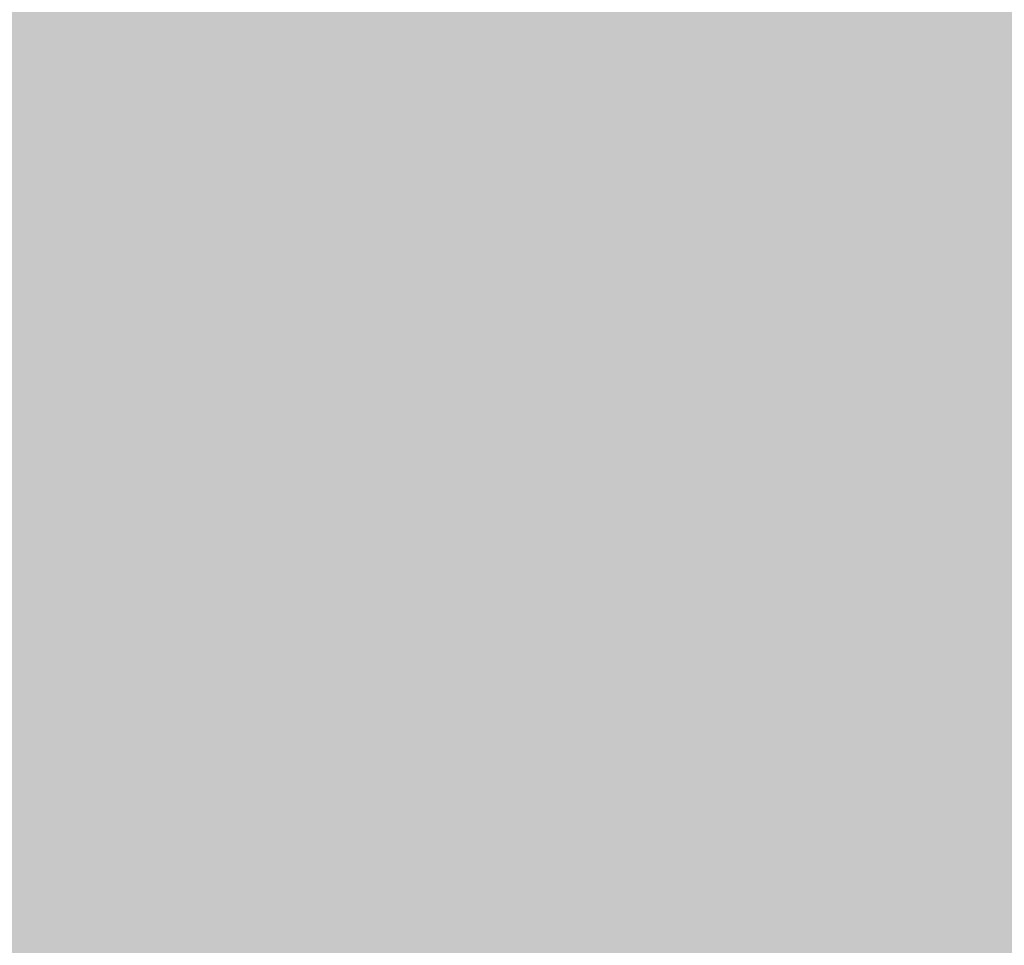
# Model space of a CAD drawing. Units: millimetres. Extents: x -22994 to 29398, y -19990 to 20176.
# Tile 86 of 135: x 227.437 to 229.428, y 85.199 to 87.071. Entities that reach past the tile are written whole.
import ezdxf
from ezdxf import colors
from ezdxf.entities.mleader import LeaderData, LeaderLine
from ezdxf.math import Vec2, Vec3

# ---------------------------------------------------------------- set-up
doc = ezdxf.new("R2010")
doc.units = ezdxf.units.MM
doc.header["$MEASUREMENT"] = 0
doc.layers.add('M-ANNO-TEXT', color=7, linetype='Continuous', lineweight=25)
doc.layers.add('M-DIMS', color=2, linetype='Continuous', lineweight=18)
doc.styles.get("Standard").update_dxf_attribs({"font": 'arial.ttf'})
doc.dimstyles.get("Standard").update_dxf_attribs({"dimtxt": 0.18, "dimasz": 10000, "dimexe": 0.18, "dimexo": 0.0625, "dimgap": 0.09, "dimtad": 0, "dimtih": 1, "dimtoh": 1, "dimdec": 0, "dimzin": 0, "dimdsep": 46, "dimtxsty": 'Standard', "dimcen": 0.09, "dimadec": 0, "dimazin": 0, "dimtfac": 1, "dimtdec": 0, "dimtofl": 0, "dimtmove": 0, "dimatfit": 3, "dimfxl": 1, "dimtolj": 1, "dimtzin": 0, "dimlwd": 30, "dimarcsym": 0})

# ---------------------------------------------------------------- blocks, each defined once
blk = doc.blocks.new('*D2')
at = {"layer": 'Defpoints', "color": 0, "transparency": 16777216}
for p in [(6.6773, 10.2713), (290.852, 10.2713), (290.852, -5.0787)]:
    blk.add_point(p, dxfattribs=at)
at = {"layer": 'M-DIMS', "color": 0, "lineweight": -2, "transparency": 16777216}
for p, q in [((6.6773, 10.2088), (6.6773, -5.2587)), ((290.852, 10.2088), (290.852, -5.2587))]:
    blk.add_line(p, q, dxfattribs=at)
at = {"layer": 'M-DIMS', "color": 0, "lineweight": 30, "transparency": 16777216}
for p, q in [((-9993.3227, -5.0787), (-19993.3227, -5.0787)), ((10290.852, -5.0787), (20290.852, -5.0787))]:
    blk.add_line(p, q, dxfattribs=at)
at = {"layer": 'M-DIMS', "color": 0, "transparency": 16777216}
for points in [[(-9993.3227, 1661.5879), (-9993.3227, -1671.7454), (6.6773, -5.0787)], [(10290.852, 1661.5879), (10290.852, -1671.7454), (290.852, -5.0787)]]:
    blk.add_solid(points, dxfattribs=at)
at = {"layer": 'M-DIMS', "color": 0, "transparency": 16777216, "insert": (148.7647, -5.0787), "char_height": 0.18, "attachment_point": 5}
blk.add_mtext('\\A1;284.2', dxfattribs=at)
blk = doc.blocks.new('*D3')
at = {"layer": 'Defpoints', "color": 0, "transparency": 16777216}
for p in [(110.2647, 204.1654), (110.2647, 176.3662), (95.8327, 127.967)]:
    blk.add_point(p, dxfattribs=at)
at = {"layer": 'M-DIMS', "color": 0, "lineweight": -2, "transparency": 16777216}
for p, q in [((95.8327, 128.0295), (95.8327, 204.3454)), ((110.2647, 176.4287), (110.2647, 204.3454))]:
    blk.add_line(p, q, dxfattribs=at)
at = {"layer": 'M-DIMS', "color": 0, "lineweight": 30, "transparency": 16777216}
for p, q in [((-9904.1673, 204.1654), (-19904.1673, 204.1654)), ((10110.2647, 204.1654), (20110.2647, 204.1654))]:
    blk.add_line(p, q, dxfattribs=at)
at = {"layer": 'M-DIMS', "color": 0, "transparency": 16777216}
for points in [[(-9904.1673, 1870.8321), (-9904.1673, -1462.5013), (95.8327, 204.1654)], [(10110.2647, 1870.8321), (10110.2647, -1462.5013), (110.2647, 204.1654)]]:
    blk.add_solid(points, dxfattribs=at)
at = {"layer": 'M-DIMS', "color": 0, "transparency": 16777216, "insert": (103.0487, 204.1654), "char_height": 0.18, "attachment_point": 5}
blk.add_mtext('\\A1;14.432', dxfattribs=at)
blk = doc.blocks.new('*D4')
at = {"layer": 'Defpoints', "color": 0, "transparency": 16777216}
for p in [(116.2647, 204.1654), (110.2647, 176.3662), (116.2647, 176.3662)]:
    blk.add_point(p, dxfattribs=at)
at = {"layer": 'M-DIMS', "color": 0, "lineweight": -2, "transparency": 16777216}
for p, q in [((110.2647, 176.4287), (110.2647, 204.3454)), ((116.2647, 176.4287), (116.2647, 204.3454))]:
    blk.add_line(p, q, dxfattribs=at)
at = {"layer": 'M-DIMS', "color": 0, "lineweight": 30, "transparency": 16777216}
for p, q in [((-9889.7353, 204.1654), (-19889.7353, 204.1654)), ((10116.2647, 204.1654), (20116.2647, 204.1654))]:
    blk.add_line(p, q, dxfattribs=at)
at = {"layer": 'M-DIMS', "color": 0, "transparency": 16777216}
for points in [[(-9889.7353, 1870.8321), (-9889.7353, -1462.5013), (110.2647, 204.1654)], [(10116.2647, 1870.8321), (10116.2647, -1462.5013), (116.2647, 204.1654)]]:
    blk.add_solid(points, dxfattribs=at)
at = {"layer": 'M-DIMS', "color": 0, "transparency": 16777216, "insert": (113.2647, 204.1654), "char_height": 0.18, "attachment_point": 5}
blk.add_mtext('\\A1;6', dxfattribs=at)
blk = doc.blocks.new('*D5')
at = {"layer": 'Defpoints', "color": 0, "transparency": 16777216}
for p in [(181.2647, 204.1654), (116.2647, 176.3662), (181.2647, 176.3662)]:
    blk.add_point(p, dxfattribs=at)
at = {"layer": 'M-DIMS', "color": 0, "lineweight": -2, "transparency": 16777216}
for p, q in [((116.2647, 176.4287), (116.2647, 204.3454)), ((181.2647, 176.4287), (181.2647, 204.3454))]:
    blk.add_line(p, q, dxfattribs=at)
at = {"layer": 'M-DIMS', "color": 0, "lineweight": 30, "transparency": 16777216}
for p, q in [((-9883.7353, 204.1654), (-19883.7353, 204.1654)), ((10181.2647, 204.1654), (20181.2647, 204.1654))]:
    blk.add_line(p, q, dxfattribs=at)
at = {"layer": 'M-DIMS', "color": 0, "transparency": 16777216}
for points in [[(-9883.7353, 1870.8321), (-9883.7353, -1462.5013), (116.2647, 204.1654)], [(10181.2647, 1870.8321), (10181.2647, -1462.5013), (181.2647, 204.1654)]]:
    blk.add_solid(points, dxfattribs=at)
at = {"layer": 'M-DIMS', "color": 0, "transparency": 16777216, "insert": (148.7647, 204.1654), "char_height": 0.18, "attachment_point": 5}
blk.add_mtext('\\A1;65', dxfattribs=at)
blk = doc.blocks.new('*D6')
at = {"layer": 'Defpoints', "color": 0, "transparency": 16777216}
for p in [(187.2647, 204.1654), (181.2647, 176.3662), (187.2647, 176.3662)]:
    blk.add_point(p, dxfattribs=at)
at = {"layer": 'M-DIMS', "color": 0, "lineweight": -2, "transparency": 16777216}
for p, q in [((181.2647, 176.4287), (181.2647, 204.3454)), ((187.2647, 176.4287), (187.2647, 204.3454))]:
    blk.add_line(p, q, dxfattribs=at)
at = {"layer": 'M-DIMS', "color": 0, "lineweight": 30, "transparency": 16777216}
for p, q in [((-9818.7353, 204.1654), (-19818.7353, 204.1654)), ((10187.2647, 204.1654), (20187.2647, 204.1654))]:
    blk.add_line(p, q, dxfattribs=at)
at = {"layer": 'M-DIMS', "color": 0, "transparency": 16777216}
for points in [[(-9818.7353, 1870.8321), (-9818.7353, -1462.5013), (181.2647, 204.1654)], [(10187.2647, 1870.8321), (10187.2647, -1462.5013), (187.2647, 204.1654)]]:
    blk.add_solid(points, dxfattribs=at)
at = {"layer": 'M-DIMS', "color": 0, "transparency": 16777216, "insert": (184.2647, 204.1654), "char_height": 0.18, "attachment_point": 5}
blk.add_mtext('\\A1;6', dxfattribs=at)
blk = doc.blocks.new('*D7')
at = {"layer": 'Defpoints', "color": 0, "transparency": 16777216}
for p in [(201.6967, 204.1654), (187.2647, 176.3662), (201.6967, 127.967)]:
    blk.add_point(p, dxfattribs=at)
at = {"layer": 'M-DIMS', "color": 0, "lineweight": -2, "transparency": 16777216}
for p, q in [((187.2647, 176.4287), (187.2647, 204.3454)), ((201.6967, 128.0295), (201.6967, 204.3454))]:
    blk.add_line(p, q, dxfattribs=at)
at = {"layer": 'M-DIMS', "color": 0, "lineweight": 30, "transparency": 16777216}
for p, q in [((-9812.7353, 204.1654), (-19812.7353, 204.1654)), ((10201.6967, 204.1654), (20201.6967, 204.1654))]:
    blk.add_line(p, q, dxfattribs=at)
at = {"layer": 'M-DIMS', "color": 0, "transparency": 16777216}
for points in [[(-9812.7353, 1870.8321), (-9812.7353, -1462.5013), (187.2647, 204.1654)], [(10201.6967, 1870.8321), (10201.6967, -1462.5013), (201.6967, 204.1654)]]:
    blk.add_solid(points, dxfattribs=at)
at = {"layer": 'M-DIMS', "color": 0, "transparency": 16777216, "insert": (194.4807, 204.1654), "char_height": 0.18, "attachment_point": 5}
blk.add_mtext('\\A1;14.432', dxfattribs=at)
blk = doc.blocks.new('*D8')
at = {"layer": 'Defpoints', "color": 0, "transparency": 16777216}
for p in [(227.6485, 204.1654), (227.6485, 146.7296), (201.6967, 127.967)]:
    blk.add_point(p, dxfattribs=at)
at = {"layer": 'M-DIMS', "color": 0, "lineweight": -2, "transparency": 16777216}
for p, q in [((201.6967, 128.0295), (201.6967, 204.3454)), ((227.6485, 146.7921), (227.6485, 204.3454))]:
    blk.add_line(p, q, dxfattribs=at)
at = {"layer": 'M-DIMS', "color": 0, "lineweight": 30, "transparency": 16777216}
for p, q in [((-9798.3033, 204.1654), (-19798.3033, 204.1654)), ((10227.6485, 204.1654), (20227.6485, 204.1654))]:
    blk.add_line(p, q, dxfattribs=at)
at = {"layer": 'M-DIMS', "color": 0, "transparency": 16777216}
for points in [[(-9798.3033, 1870.8321), (-9798.3033, -1462.5013), (201.6967, 204.1654)], [(10227.6485, 1870.8321), (10227.6485, -1462.5013), (227.6485, 204.1654)]]:
    blk.add_solid(points, dxfattribs=at)
at = {"layer": 'M-DIMS', "color": 0, "transparency": 16777216, "insert": (214.6726, 204.1654), "char_height": 0.18, "attachment_point": 5}
blk.add_mtext('\\A1;25.95', dxfattribs=at)
blk = doc.blocks.new('*D9')
at = {"layer": 'Defpoints', "color": 0, "transparency": 16777216}
for p in [(187.2647, 176.3662), (306.202, 176.3662), (290.852, 10.2713)]:
    blk.add_point(p, dxfattribs=at)
at = {"layer": 'M-DIMS', "color": 0, "lineweight": 30, "transparency": 16777216}
for p, q in [((306.202, 10176.3662), (306.202, 20176.3662)), ((306.202, -9989.7287), (306.202, -19989.7287))]:
    blk.add_line(p, q, dxfattribs=at)
at = {"layer": 'M-DIMS', "color": 0, "lineweight": -2, "transparency": 16777216}
for p, q in [((187.3272, 176.3662), (306.382, 176.3662)), ((290.9145, 10.2713), (306.382, 10.2713))]:
    blk.add_line(p, q, dxfattribs=at)
at = {"layer": 'M-DIMS', "color": 0, "transparency": 16777216}
for points in [[(-1360.4646, 10176.3662), (1972.8687, 10176.3662), (306.202, 176.3662)], [(-1360.4646, -9989.7287), (1972.8687, -9989.7287), (306.202, 10.2713)]]:
    blk.add_solid(points, dxfattribs=at)
at = {"layer": 'M-DIMS', "color": 0, "transparency": 16777216, "insert": (306.202, 93.3187), "char_height": 0.18, "attachment_point": 5}
blk.add_mtext('\\A1;166.1', dxfattribs=at)
blk = doc.blocks.new('*D10')
at = {"layer": 'Defpoints', "color": 0, "transparency": 16777216}
for p in [(125.6498, 136.0713), (133.3459, 136.0713), (133.3459, -5.0787)]:
    blk.add_point(p, dxfattribs=at)
at = {"layer": 'M-DIMS', "color": 0, "lineweight": -2, "transparency": 16777216}
for p, q in [((125.6498, 136.0088), (125.6498, -5.2587)), ((133.3459, 136.0088), (133.3459, -5.2587))]:
    blk.add_line(p, q, dxfattribs=at)
at = {"layer": 'M-DIMS', "color": 0, "lineweight": 30, "transparency": 16777216}
for p, q in [((-9874.3502, -5.0787), (-19874.3502, -5.0787)), ((10133.3459, -5.0787), (20133.3459, -5.0787))]:
    blk.add_line(p, q, dxfattribs=at)
at = {"layer": 'M-DIMS', "color": 0, "transparency": 16777216}
for points in [[(-9874.3502, 1661.5879), (-9874.3502, -1671.7454), (125.6498, -5.0787)], [(10133.3459, 1661.5879), (10133.3459, -1671.7454), (133.3459, -5.0787)]]:
    blk.add_solid(points, dxfattribs=at)
at = {"layer": 'M-DIMS', "color": 0, "transparency": 16777216, "insert": (129.4978, -5.0787), "char_height": 0.18, "attachment_point": 5}
blk.add_mtext('\\A1;7.696', dxfattribs=at)
blk = doc.blocks.new('*D11')
at = {"layer": 'Defpoints', "color": 0, "transparency": 16777216}
for p in [(133.3459, 136.0713), (135.6498, 136.0713), (135.6498, -5.0787)]:
    blk.add_point(p, dxfattribs=at)
at = {"layer": 'M-DIMS', "color": 0, "lineweight": -2, "transparency": 16777216}
for p, q in [((133.3459, 136.0088), (133.3459, -5.2587)), ((135.6498, 136.0088), (135.6498, -5.2587))]:
    blk.add_line(p, q, dxfattribs=at)
at = {"layer": 'M-DIMS', "color": 0, "lineweight": 30, "transparency": 16777216}
for p, q in [((-9866.6541, -5.0787), (-19866.6541, -5.0787)), ((10135.6498, -5.0787), (20135.6498, -5.0787))]:
    blk.add_line(p, q, dxfattribs=at)
at = {"layer": 'M-DIMS', "color": 0, "transparency": 16777216}
for points in [[(-9866.6541, 1661.5879), (-9866.6541, -1671.7454), (133.3459, -5.0787)], [(10135.6498, 1661.5879), (10135.6498, -1671.7454), (135.6498, -5.0787)]]:
    blk.add_solid(points, dxfattribs=at)
at = {"layer": 'M-DIMS', "color": 0, "transparency": 16777216, "insert": (134.4978, -5.0787), "char_height": 0.18, "attachment_point": 5}
blk.add_mtext('\\A1;2.304', dxfattribs=at)
blk = doc.blocks.new('*D12')
at = {"layer": 'Defpoints', "color": 0, "transparency": 16777216}
for p in [(135.6498, 136.0713), (145.6498, 136.0713), (145.6498, -5.0787)]:
    blk.add_point(p, dxfattribs=at)
at = {"layer": 'M-DIMS', "color": 0, "lineweight": -2, "transparency": 16777216}
for p, q in [((135.6498, 136.0088), (135.6498, -5.2587)), ((145.6498, 136.0088), (145.6498, -5.2587))]:
    blk.add_line(p, q, dxfattribs=at)
at = {"layer": 'M-DIMS', "color": 0, "lineweight": 30, "transparency": 16777216}
for p, q in [((-9864.3502, -5.0787), (-19864.3502, -5.0787)), ((10145.6498, -5.0787), (20145.6498, -5.0787))]:
    blk.add_line(p, q, dxfattribs=at)
at = {"layer": 'M-DIMS', "color": 0, "transparency": 16777216}
for points in [[(-9864.3502, 1661.5879), (-9864.3502, -1671.7454), (135.6498, -5.0787)], [(10145.6498, 1661.5879), (10145.6498, -1671.7454), (145.6498, -5.0787)]]:
    blk.add_solid(points, dxfattribs=at)
at = {"layer": 'M-DIMS', "color": 0, "transparency": 16777216, "insert": (140.6498, -5.0787), "char_height": 0.18, "attachment_point": 5}
blk.add_mtext('\\A1;10', dxfattribs=at)
blk = doc.blocks.new('*D13')
at = {"layer": 'Defpoints', "color": 0, "transparency": 16777216}
for p in [(145.6498, 136.0713), (155.6498, 136.0713), (155.6498, -5.0787)]:
    blk.add_point(p, dxfattribs=at)
at = {"layer": 'M-DIMS', "color": 0, "lineweight": -2, "transparency": 16777216}
for p, q in [((145.6498, 136.0088), (145.6498, -5.2587)), ((155.6498, 136.0088), (155.6498, -5.2587))]:
    blk.add_line(p, q, dxfattribs=at)
at = {"layer": 'M-DIMS', "color": 0, "lineweight": 30, "transparency": 16777216}
for p, q in [((-9854.3502, -5.0787), (-19854.3502, -5.0787)), ((10155.6498, -5.0787), (20155.6498, -5.0787))]:
    blk.add_line(p, q, dxfattribs=at)
at = {"layer": 'M-DIMS', "color": 0, "transparency": 16777216}
for points in [[(-9854.3502, 1661.5879), (-9854.3502, -1671.7454), (145.6498, -5.0787)], [(10155.6498, 1661.5879), (10155.6498, -1671.7454), (155.6498, -5.0787)]]:
    blk.add_solid(points, dxfattribs=at)
at = {"layer": 'M-DIMS', "color": 0, "transparency": 16777216, "insert": (150.6498, -5.0787), "char_height": 0.18, "attachment_point": 5}
blk.add_mtext('\\A1;10', dxfattribs=at)
blk = doc.blocks.new('*D14')
at = {"layer": 'Defpoints', "color": 0, "transparency": 16777216}
for p in [(155.6498, 136.0713), (165.6498, 136.0713), (165.6498, -5.0787)]:
    blk.add_point(p, dxfattribs=at)
at = {"layer": 'M-DIMS', "color": 0, "lineweight": -2, "transparency": 16777216}
for p, q in [((155.6498, 136.0088), (155.6498, -5.2587)), ((165.6498, 136.0088), (165.6498, -5.2587))]:
    blk.add_line(p, q, dxfattribs=at)
at = {"layer": 'M-DIMS', "color": 0, "lineweight": 30, "transparency": 16777216}
for p, q in [((-9844.3502, -5.0787), (-19844.3502, -5.0787)), ((10165.6498, -5.0787), (20165.6498, -5.0787))]:
    blk.add_line(p, q, dxfattribs=at)
at = {"layer": 'M-DIMS', "color": 0, "transparency": 16777216}
for points in [[(-9844.3502, 1661.5879), (-9844.3502, -1671.7454), (155.6498, -5.0787)], [(10165.6498, 1661.5879), (10165.6498, -1671.7454), (165.6498, -5.0787)]]:
    blk.add_solid(points, dxfattribs=at)
at = {"layer": 'M-DIMS', "color": 0, "transparency": 16777216, "insert": (160.6498, -5.0787), "char_height": 0.18, "attachment_point": 5}
blk.add_mtext('\\A1;10', dxfattribs=at)
blk = doc.blocks.new('*D15')
at = {"layer": 'Defpoints', "color": 0, "transparency": 16777216}
for p in [(173.3459, 154.788), (173.3459, 136.0713), (306.202, 136.0713)]:
    blk.add_point(p, dxfattribs=at)
at = {"layer": 'M-DIMS', "color": 0, "lineweight": 30, "transparency": 16777216}
for p, q in [((306.202, 10154.788), (306.202, 20154.788)), ((306.202, -9863.9287), (306.202, -19863.9287))]:
    blk.add_line(p, q, dxfattribs=at)
at = {"layer": 'M-DIMS', "color": 0, "lineweight": -2, "transparency": 16777216}
for p, q in [((173.4084, 154.788), (306.382, 154.788)), ((173.4084, 136.0713), (306.382, 136.0713))]:
    blk.add_line(p, q, dxfattribs=at)
at = {"layer": 'M-DIMS', "color": 0, "transparency": 16777216}
for points in [[(-1360.4646, 10154.788), (1972.8687, 10154.788), (306.202, 154.788)], [(-1360.4646, -9863.9287), (1972.8687, -9863.9287), (306.202, 136.0713)]]:
    blk.add_solid(points, dxfattribs=at)
at = {"layer": 'M-DIMS', "color": 0, "transparency": 16777216, "insert": (306.202, 145.4297), "char_height": 0.18, "attachment_point": 5}
blk.add_mtext('\\A1;18.717', dxfattribs=at)
blk = doc.blocks.new('*D16')
at = {"layer": 'Defpoints', "color": 0, "transparency": 16777216}
for p in [(120.1702, 204.1654), (110.4658, 48.0349), (120.1702, 48.0349)]:
    blk.add_point(p, dxfattribs=at)
at = {"layer": 'M-DIMS', "color": 0, "lineweight": -2, "transparency": 16777216}
for p, q in [((110.4658, 48.0974), (110.4658, 204.3454)), ((120.1702, 48.0974), (120.1702, 204.3454))]:
    blk.add_line(p, q, dxfattribs=at)
at = {"layer": 'M-DIMS', "color": 0, "lineweight": 30, "transparency": 16777216}
for p, q in [((-9889.5342, 204.1654), (-19889.5342, 204.1654)), ((10120.1702, 204.1654), (20120.1702, 204.1654))]:
    blk.add_line(p, q, dxfattribs=at)
at = {"layer": 'M-DIMS', "color": 0, "transparency": 16777216}
for points in [[(-9889.5342, 1870.8321), (-9889.5342, -1462.5013), (110.4658, 204.1654)], [(10120.1702, 1870.8321), (10120.1702, -1462.5013), (120.1702, 204.1654)]]:
    blk.add_solid(points, dxfattribs=at)
at = {"layer": 'M-DIMS', "color": 0, "transparency": 16777216, "insert": (115.318, 204.1654), "char_height": 0.18, "attachment_point": 5}
blk.add_mtext('\\A1;9.704', dxfattribs=at)
blk = doc.blocks.new('*D17')
at = {"layer": 'Defpoints', "color": 0, "transparency": 16777216}
for p in [(126.1702, 204.1654), (120.1702, 48.0349), (126.1702, 48.0349)]:
    blk.add_point(p, dxfattribs=at)
at = {"layer": 'M-DIMS', "color": 0, "lineweight": -2, "transparency": 16777216}
for p, q in [((120.1702, 48.0974), (120.1702, 204.3454)), ((126.1702, 48.0974), (126.1702, 204.3454))]:
    blk.add_line(p, q, dxfattribs=at)
at = {"layer": 'M-DIMS', "color": 0, "lineweight": 30, "transparency": 16777216}
for p, q in [((-9879.8298, 204.1654), (-19879.8298, 204.1654)), ((10126.1702, 204.1654), (20126.1702, 204.1654))]:
    blk.add_line(p, q, dxfattribs=at)
at = {"layer": 'M-DIMS', "color": 0, "transparency": 16777216}
for points in [[(-9879.8298, 1870.8321), (-9879.8298, -1462.5013), (120.1702, 204.1654)], [(10126.1702, 1870.8321), (10126.1702, -1462.5013), (126.1702, 204.1654)]]:
    blk.add_solid(points, dxfattribs=at)
at = {"layer": 'M-DIMS', "color": 0, "transparency": 16777216, "insert": (123.1702, 204.1654), "char_height": 0.18, "attachment_point": 5}
blk.add_mtext('\\A1;6', dxfattribs=at)
blk = doc.blocks.new('*D18')
at = {"layer": 'Defpoints', "color": 0, "transparency": 16777216}
for p in [(132.1702, 204.1654), (126.1702, 48.0349), (132.1702, 48.0349)]:
    blk.add_point(p, dxfattribs=at)
at = {"layer": 'M-DIMS', "color": 0, "lineweight": -2, "transparency": 16777216}
for p, q in [((126.1702, 48.0974), (126.1702, 204.3454)), ((132.1702, 48.0974), (132.1702, 204.3454))]:
    blk.add_line(p, q, dxfattribs=at)
at = {"layer": 'M-DIMS', "color": 0, "lineweight": 30, "transparency": 16777216}
for p, q in [((-9873.8298, 204.1654), (-19873.8298, 204.1654)), ((10132.1702, 204.1654), (20132.1702, 204.1654))]:
    blk.add_line(p, q, dxfattribs=at)
at = {"layer": 'M-DIMS', "color": 0, "transparency": 16777216}
for points in [[(-9873.8298, 1870.8321), (-9873.8298, -1462.5013), (126.1702, 204.1654)], [(10132.1702, 1870.8321), (10132.1702, -1462.5013), (132.1702, 204.1654)]]:
    blk.add_solid(points, dxfattribs=at)
at = {"layer": 'M-DIMS', "color": 0, "transparency": 16777216, "insert": (129.1702, 204.1654), "char_height": 0.18, "attachment_point": 5}
blk.add_mtext('\\A1;6', dxfattribs=at)
blk = doc.blocks.new('*D19')
at = {"layer": 'Defpoints', "color": 0, "transparency": 16777216}
for p in [(138.1702, 204.1654), (132.1702, 48.0349), (138.1702, 48.0349)]:
    blk.add_point(p, dxfattribs=at)
at = {"layer": 'M-DIMS', "color": 0, "lineweight": -2, "transparency": 16777216}
for p, q in [((132.1702, 48.0974), (132.1702, 204.3454)), ((138.1702, 48.0974), (138.1702, 204.3454))]:
    blk.add_line(p, q, dxfattribs=at)
at = {"layer": 'M-DIMS', "color": 0, "lineweight": 30, "transparency": 16777216}
for p, q in [((-9867.8298, 204.1654), (-19867.8298, 204.1654)), ((10138.1702, 204.1654), (20138.1702, 204.1654))]:
    blk.add_line(p, q, dxfattribs=at)
at = {"layer": 'M-DIMS', "color": 0, "transparency": 16777216}
for points in [[(-9867.8298, 1870.8321), (-9867.8298, -1462.5013), (132.1702, 204.1654)], [(10138.1702, 1870.8321), (10138.1702, -1462.5013), (138.1702, 204.1654)]]:
    blk.add_solid(points, dxfattribs=at)
at = {"layer": 'M-DIMS', "color": 0, "transparency": 16777216, "insert": (135.1702, 204.1654), "char_height": 0.18, "attachment_point": 5}
blk.add_mtext('\\A1;6', dxfattribs=at)
blk = doc.blocks.new('*D20')
at = {"layer": 'Defpoints', "color": 0, "transparency": 16777216}
for p in [(144.1702, 204.1654), (138.1702, 48.0349), (144.1702, 48.0349)]:
    blk.add_point(p, dxfattribs=at)
at = {"layer": 'M-DIMS', "color": 0, "lineweight": -2, "transparency": 16777216}
for p, q in [((138.1702, 48.0974), (138.1702, 204.3454)), ((144.1702, 48.0974), (144.1702, 204.3454))]:
    blk.add_line(p, q, dxfattribs=at)
at = {"layer": 'M-DIMS', "color": 0, "lineweight": 30, "transparency": 16777216}
for p, q in [((-9861.8298, 204.1654), (-19861.8298, 204.1654)), ((10144.1702, 204.1654), (20144.1702, 204.1654))]:
    blk.add_line(p, q, dxfattribs=at)
at = {"layer": 'M-DIMS', "color": 0, "transparency": 16777216}
for points in [[(-9861.8298, 1870.8321), (-9861.8298, -1462.5013), (138.1702, 204.1654)], [(10144.1702, 1870.8321), (10144.1702, -1462.5013), (144.1702, 204.1654)]]:
    blk.add_solid(points, dxfattribs=at)
at = {"layer": 'M-DIMS', "color": 0, "transparency": 16777216, "insert": (141.1702, 204.1654), "char_height": 0.18, "attachment_point": 5}
blk.add_mtext('\\A1;6', dxfattribs=at)
blk = doc.blocks.new('*D21')
at = {"layer": 'Defpoints', "color": 0, "transparency": 16777216}
for p in [(149.1157, 204.1654), (144.1702, 48.0349), (149.1157, 48.0349)]:
    blk.add_point(p, dxfattribs=at)
at = {"layer": 'M-DIMS', "color": 0, "lineweight": -2, "transparency": 16777216}
for p, q in [((144.1702, 48.0974), (144.1702, 204.3454)), ((149.1157, 48.0974), (149.1157, 204.3454))]:
    blk.add_line(p, q, dxfattribs=at)
at = {"layer": 'M-DIMS', "color": 0, "lineweight": 30, "transparency": 16777216}
for p, q in [((-9855.8298, 204.1654), (-19855.8298, 204.1654)), ((10149.1157, 204.1654), (20149.1157, 204.1654))]:
    blk.add_line(p, q, dxfattribs=at)
at = {"layer": 'M-DIMS', "color": 0, "transparency": 16777216}
for points in [[(-9855.8298, 1870.8321), (-9855.8298, -1462.5013), (144.1702, 204.1654)], [(10149.1157, 1870.8321), (10149.1157, -1462.5013), (149.1157, 204.1654)]]:
    blk.add_solid(points, dxfattribs=at)
at = {"layer": 'M-DIMS', "color": 0, "transparency": 16777216, "insert": (146.6429, 204.1654), "char_height": 0.18, "attachment_point": 5}
blk.add_mtext('\\A1;4.945', dxfattribs=at)
blk = doc.blocks.new('*D22')
at = {"layer": 'Defpoints', "color": 0, "transparency": 16777216}
for p in [(149.1157, 30.9895), (155.1157, 30.9895), (155.1157, -5.0787)]:
    blk.add_point(p, dxfattribs=at)
at = {"layer": 'M-DIMS', "color": 0, "lineweight": -2, "transparency": 16777216}
for p, q in [((149.1157, 30.927), (149.1157, -5.2587)), ((155.1157, 30.927), (155.1157, -5.2587))]:
    blk.add_line(p, q, dxfattribs=at)
at = {"layer": 'M-DIMS', "color": 0, "lineweight": 30, "transparency": 16777216}
for p, q in [((-9850.8843, -5.0787), (-19850.8843, -5.0787)), ((10155.1157, -5.0787), (20155.1157, -5.0787))]:
    blk.add_line(p, q, dxfattribs=at)
at = {"layer": 'M-DIMS', "color": 0, "transparency": 16777216}
for points in [[(-9850.8843, 1661.5879), (-9850.8843, -1671.7454), (149.1157, -5.0787)], [(10155.1157, 1661.5879), (10155.1157, -1671.7454), (155.1157, -5.0787)]]:
    blk.add_solid(points, dxfattribs=at)
at = {"layer": 'M-DIMS', "color": 0, "transparency": 16777216, "insert": (152.1157, -5.0787), "char_height": 0.18, "attachment_point": 5}
blk.add_mtext('\\A1;6', dxfattribs=at)
blk = doc.blocks.new('*D23')
at = {"layer": 'Defpoints', "color": 0, "transparency": 16777216}
for p in [(155.1157, 30.9895), (161.1157, 30.9895), (161.1157, -5.0787)]:
    blk.add_point(p, dxfattribs=at)
at = {"layer": 'M-DIMS', "color": 0, "lineweight": -2, "transparency": 16777216}
for p, q in [((155.1157, 30.927), (155.1157, -5.2587)), ((161.1157, 30.927), (161.1157, -5.2587))]:
    blk.add_line(p, q, dxfattribs=at)
at = {"layer": 'M-DIMS', "color": 0, "lineweight": 30, "transparency": 16777216}
for p, q in [((-9844.8843, -5.0787), (-19844.8843, -5.0787)), ((10161.1157, -5.0787), (20161.1157, -5.0787))]:
    blk.add_line(p, q, dxfattribs=at)
at = {"layer": 'M-DIMS', "color": 0, "transparency": 16777216}
for points in [[(-9844.8843, 1661.5879), (-9844.8843, -1671.7454), (155.1157, -5.0787)], [(10161.1157, 1661.5879), (10161.1157, -1671.7454), (161.1157, -5.0787)]]:
    blk.add_solid(points, dxfattribs=at)
at = {"layer": 'M-DIMS', "color": 0, "transparency": 16777216, "insert": (158.1157, -5.0787), "char_height": 0.18, "attachment_point": 5}
blk.add_mtext('\\A1;6', dxfattribs=at)
blk = doc.blocks.new('*D24')
at = {"layer": 'Defpoints', "color": 0, "transparency": 16777216}
for p in [(161.1157, 30.9895), (166.4387, 30.9895), (166.4387, -5.0787)]:
    blk.add_point(p, dxfattribs=at)
at = {"layer": 'M-DIMS', "color": 0, "lineweight": -2, "transparency": 16777216}
for p, q in [((161.1157, 30.927), (161.1157, -5.2587)), ((166.4387, 30.927), (166.4387, -5.2587))]:
    blk.add_line(p, q, dxfattribs=at)
at = {"layer": 'M-DIMS', "color": 0, "lineweight": 30, "transparency": 16777216}
for p, q in [((-9838.8843, -5.0787), (-19838.8843, -5.0787)), ((10166.4387, -5.0787), (20166.4387, -5.0787))]:
    blk.add_line(p, q, dxfattribs=at)
at = {"layer": 'M-DIMS', "color": 0, "transparency": 16777216}
for points in [[(-9838.8843, 1661.5879), (-9838.8843, -1671.7454), (161.1157, -5.0787)], [(10166.4387, 1661.5879), (10166.4387, -1671.7454), (166.4387, -5.0787)]]:
    blk.add_solid(points, dxfattribs=at)
at = {"layer": 'M-DIMS', "color": 0, "transparency": 16777216, "insert": (163.7772, -5.0787), "char_height": 0.18, "attachment_point": 5}
blk.add_mtext('\\A1;5.323', dxfattribs=at)
blk = doc.blocks.new('*D25')
at = {"layer": 'Defpoints', "color": 0, "transparency": 16777216}
for p in [(166.4387, 30.9895), (172.4387, 30.9895), (172.4387, -5.0787)]:
    blk.add_point(p, dxfattribs=at)
at = {"layer": 'M-DIMS', "color": 0, "lineweight": -2, "transparency": 16777216}
for p, q in [((166.4387, 30.927), (166.4387, -5.2587)), ((172.4387, 30.927), (172.4387, -5.2587))]:
    blk.add_line(p, q, dxfattribs=at)
at = {"layer": 'M-DIMS', "color": 0, "lineweight": 30, "transparency": 16777216}
for p, q in [((-9833.5613, -5.0787), (-19833.5613, -5.0787)), ((10172.4387, -5.0787), (20172.4387, -5.0787))]:
    blk.add_line(p, q, dxfattribs=at)
at = {"layer": 'M-DIMS', "color": 0, "transparency": 16777216}
for points in [[(-9833.5613, 1661.5879), (-9833.5613, -1671.7454), (166.4387, -5.0787)], [(10172.4387, 1661.5879), (10172.4387, -1671.7454), (172.4387, -5.0787)]]:
    blk.add_solid(points, dxfattribs=at)
at = {"layer": 'M-DIMS', "color": 0, "transparency": 16777216, "insert": (169.4387, -5.0787), "char_height": 0.18, "attachment_point": 5}
blk.add_mtext('\\A1;6', dxfattribs=at)
blk = doc.blocks.new('*D26')
at = {"layer": 'Defpoints', "color": 0, "transparency": 16777216}
for p in [(172.4387, 30.9895), (178.4387, 30.9895), (178.4387, -5.0787)]:
    blk.add_point(p, dxfattribs=at)
at = {"layer": 'M-DIMS', "color": 0, "lineweight": -2, "transparency": 16777216}
for p, q in [((172.4387, 30.927), (172.4387, -5.2587)), ((178.4387, 30.927), (178.4387, -5.2587))]:
    blk.add_line(p, q, dxfattribs=at)
at = {"layer": 'M-DIMS', "color": 0, "lineweight": 30, "transparency": 16777216}
for p, q in [((-9827.5613, -5.0787), (-19827.5613, -5.0787)), ((10178.4387, -5.0787), (20178.4387, -5.0787))]:
    blk.add_line(p, q, dxfattribs=at)
at = {"layer": 'M-DIMS', "color": 0, "transparency": 16777216}
for points in [[(-9827.5613, 1661.5879), (-9827.5613, -1671.7454), (172.4387, -5.0787)], [(10178.4387, 1661.5879), (10178.4387, -1671.7454), (178.4387, -5.0787)]]:
    blk.add_solid(points, dxfattribs=at)
at = {"layer": 'M-DIMS', "color": 0, "transparency": 16777216, "insert": (175.4387, -5.0787), "char_height": 0.18, "attachment_point": 5}
blk.add_mtext('\\A1;6', dxfattribs=at)
blk = doc.blocks.new('*D27')
at = {"layer": 'Defpoints', "color": 0, "transparency": 16777216}
for p in [(178.4387, 30.9895), (188.1175, 30.9895), (188.1175, -5.0787)]:
    blk.add_point(p, dxfattribs=at)
at = {"layer": 'M-DIMS', "color": 0, "lineweight": -2, "transparency": 16777216}
for p, q in [((178.4387, 30.927), (178.4387, -5.2587)), ((188.1175, 30.927), (188.1175, -5.2587))]:
    blk.add_line(p, q, dxfattribs=at)
at = {"layer": 'M-DIMS', "color": 0, "lineweight": 30, "transparency": 16777216}
for p, q in [((-9821.5613, -5.0787), (-19821.5613, -5.0787)), ((10188.1175, -5.0787), (20188.1175, -5.0787))]:
    blk.add_line(p, q, dxfattribs=at)
at = {"layer": 'M-DIMS', "color": 0, "transparency": 16777216}
for points in [[(-9821.5613, 1661.5879), (-9821.5613, -1671.7454), (178.4387, -5.0787)], [(10188.1175, 1661.5879), (10188.1175, -1671.7454), (188.1175, -5.0787)]]:
    blk.add_solid(points, dxfattribs=at)
at = {"layer": 'M-DIMS', "color": 0, "transparency": 16777216, "insert": (183.2781, -5.0787), "char_height": 0.18, "attachment_point": 5}
blk.add_mtext('\\A1;9.679', dxfattribs=at)
blk = doc.blocks.new('*D28')
at = {"layer": 'Defpoints', "color": 0, "transparency": 16777216}
for p in [(188.1175, 48.0349), (306.202, 48.0349), (188.1175, 30.9895)]:
    blk.add_point(p, dxfattribs=at)
at = {"layer": 'M-DIMS', "color": 0, "lineweight": 30, "transparency": 16777216}
for p, q in [((306.202, 10048.0349), (306.202, 20048.0349)), ((306.202, -9969.0105), (306.202, -19969.0105))]:
    blk.add_line(p, q, dxfattribs=at)
at = {"layer": 'M-DIMS', "color": 0, "lineweight": -2, "transparency": 16777216}
for p, q in [((188.18, 48.0349), (306.382, 48.0349)), ((188.18, 30.9895), (306.382, 30.9895))]:
    blk.add_line(p, q, dxfattribs=at)
at = {"layer": 'M-DIMS', "color": 0, "transparency": 16777216}
for points in [[(-1360.4646, 10048.0349), (1972.8687, 10048.0349), (306.202, 48.0349)], [(-1360.4646, -9969.0105), (1972.8687, -9969.0105), (306.202, 30.9895)]]:
    blk.add_solid(points, dxfattribs=at)
at = {"layer": 'M-DIMS', "color": 0, "transparency": 16777216, "insert": (306.202, 39.5122), "char_height": 0.18, "attachment_point": 5}
blk.add_mtext('\\A1;17.045', dxfattribs=at)
blk = doc.blocks.new('*D29')
at = {"layer": 'Defpoints', "color": 0, "transparency": 16777216}
for p in [(36.8006, 80.045), (64.0296, 80.045)]:
    blk.add_point(p, dxfattribs=at)
at = {"layer": 'M-DIMS', "color": 0, "lineweight": -2, "transparency": 16777216}
for p, q in [((50.4151, 79.955), (50.4151, 80.135)), ((50.3251, 80.045), (50.5051, 80.045))]:
    blk.add_line(p, q, dxfattribs=at)
at = {"layer": 'M-DIMS', "color": 0, "lineweight": 30, "transparency": 16777216}
blk.add_line((20064.0296, 80.0303), (10064.0296, 80.0377), dxfattribs=at)
at = {"layer": 'M-DIMS', "color": 0, "transparency": 16777216}
blk.add_solid([(10064.0309, 1746.7043), (10064.0284, -1586.629), (64.0296, 80.045)], dxfattribs=at)
at = {"layer": 'M-DIMS', "color": 0, "transparency": 16777216, "insert": (20064.5213, 80.0303), "char_height": 0.18, "attachment_point": 5}
blk.add_mtext('\\A1;∅27.23', dxfattribs=at)
blk = doc.blocks.new('*D30')
at = {"layer": 'Defpoints', "color": 0, "transparency": 16777216}
for p in [(216.3148, 146.7291), (238.9821, 146.73)]:
    blk.add_point(p, dxfattribs=at)
at = {"layer": 'M-DIMS', "color": 0, "lineweight": 30, "transparency": 16777216}
blk.add_line((20238.9821, 147.4959), (10238.9821, 147.1129), dxfattribs=at)
at = {"layer": 'M-DIMS', "color": 0, "lineweight": -2, "transparency": 16777216}
for p, q in [((227.6485, 146.6396), (227.6485, 146.8196)), ((227.5585, 146.7296), (227.7385, 146.7296))]:
    blk.add_line(p, q, dxfattribs=at)
at = {"layer": 'M-DIMS', "color": 0, "transparency": 16777216}
blk.add_solid([(10238.9183, 1813.7796), (10239.0459, -1519.5537), (238.9821, 146.73)], dxfattribs=at)
at = {"layer": 'M-DIMS', "color": 0, "transparency": 16777216, "insert": (20239.5436, 147.4959), "char_height": 0.18, "attachment_point": 5}
blk.add_mtext('\\A1;∅22.667', dxfattribs=at)
blk = doc.blocks.new('*D31')
at = {"layer": 'Defpoints', "color": 0, "transparency": 16777216}
for p in [(223.1641, 146.7291), (232.1328, 146.73)]:
    blk.add_point(p, dxfattribs=at)
at = {"layer": 'M-DIMS', "color": 0, "lineweight": 30, "transparency": 16777216}
blk.add_line((20232.1327, 148.6656), (10232.1328, 147.6978), dxfattribs=at)
at = {"layer": 'M-DIMS', "color": 0, "lineweight": -2, "transparency": 16777216}
for p, q in [((227.6485, 146.6396), (227.6485, 146.8196)), ((227.5585, 146.7296), (227.7385, 146.7296))]:
    blk.add_line(p, q, dxfattribs=at)
at = {"layer": 'M-DIMS', "color": 0, "transparency": 16777216}
blk.add_solid([(10231.9715, 1814.3645), (10232.2941, -1518.9688), (232.1328, 146.73)], dxfattribs=at)
at = {"layer": 'M-DIMS', "color": 0, "transparency": 16777216, "insert": (20232.6245, 148.6656), "char_height": 0.18, "attachment_point": 5}
blk.add_mtext('\\A1;∅8.969', dxfattribs=at)
blk = doc.blocks.new('*D36')
at = {"layer": 'Defpoints', "color": 0, "transparency": 16777216}
for p in [(46.39, 31.3035), (46.3875, 26.5934)]:
    blk.add_point(p, dxfattribs=at)
at = {"layer": 'M-DIMS', "color": 0, "lineweight": 30, "transparency": 16777216}
for p, q in [((57.1499, 20031.3006), (51.77, 10031.302)), ((10057.1499, 20031.3006), (57.1499, 20031.3006))]:
    blk.add_line(p, q, dxfattribs=at)
at = {"layer": 'M-DIMS', "color": 0, "lineweight": -2, "transparency": 16777216}
for p, q in [((46.3887, 28.8585), (46.3887, 29.0385)), ((46.2987, 28.9485), (46.4787, 28.9485))]:
    blk.add_line(p, q, dxfattribs=at)
at = {"layer": 'M-DIMS', "color": 0, "transparency": 16777216}
blk.add_solid([(-1614.8965, 10032.1987), (1718.4364, 10030.4054), (46.39, 31.3035)], dxfattribs=at)
at = {"layer": 'M-DIMS', "color": 0, "transparency": 16777216, "insert": (10057.5542, 20031.3006), "char_height": 0.18, "attachment_point": 5}
blk.add_mtext('\\A1;∅4.71', dxfattribs=at)

msp = doc.modelspace()

# ---------------------------------------------------------------- dimensions: what is measured, and where the dimension line sits
at = {"layer": 'M-DIMS'}
for base, p1, p2, override, picture, middle in [((306.202, 176.3662), (290.852, 10.2713), (187.2647, 176.3662), {"dimdec": 1, "dimlfac": 1, "dimrnd": 0, "dimzin": 0, "dimdsep": 46, "dimlunit": 2}, '*D9', (306.202, 93.3187)), ((306.202, 136.0713), (173.3459, 154.788), (173.3459, 136.0713), {"dimdec": 3, "dimlfac": 1, "dimrnd": 0, "dimzin": 0, "dimdsep": 46, "dimlunit": 2}, '*D15', (306.202, 145.4297)), ((306.202, 48.0349), (188.1175, 30.9895), (188.1175, 48.0349), {"dimdec": 3, "dimlfac": 1, "dimrnd": 0, "dimzin": 0, "dimdsep": 46, "dimlunit": 2}, '*D28', (306.202, 39.5122))]:
    dim = msp.add_linear_dim(base=base, p1=p1, p2=p2, angle=90, dimstyle='Standard', override=override, dxfattribs=at)
    dim.commit()
    dim.dimension.update_dxf_attribs({"geometry": picture, "text_midpoint": middle})
for p1, p2, override, picture, middle in [((46.3875, 26.5934), (46.39, 31.3035), {"dimdec": 2, "dimlfac": 1, "dimrnd": 0, "dimzin": 0, "dimdsep": 46, "dimlunit": 2}, '*D36', (10057.5542, 20031.3006)), ((223.1641, 146.7291), (232.1328, 146.73), {"dimdec": 3, "dimlfac": 1, "dimrnd": 0, "dimzin": 0, "dimdsep": 46, "dimlunit": 2}, '*D31', (20232.1327, 148.6656)), ((216.3148, 146.7291), (238.9821, 146.73), {"dimdec": 3, "dimlfac": 1, "dimrnd": 0, "dimzin": 0, "dimdsep": 46, "dimlunit": 2}, '*D30', (20238.9821, 147.4959))]:
    dim = msp.add_diameter_dim_2p(p1=p1, p2=p2, dimstyle='Standard', override=override, dxfattribs=at)
    dim.commit()
    dim.dimension.update_dxf_attribs({"geometry": picture, "text_midpoint": middle, "dimtype": 163})
for base, p1, p2, override, picture, middle in [((110.2647, 204.1654), (95.8327, 127.967), (110.2647, 176.3662), {"dimdec": 3, "dimlfac": 1, "dimrnd": 0, "dimzin": 0, "dimdsep": 46, "dimlunit": 2}, '*D3', (103.0487, 204.1654)), ((116.2647, 204.1654), (110.2647, 176.3662), (116.2647, 176.3662), {"dimdec": 0, "dimlfac": 1, "dimrnd": 0, "dimzin": 0, "dimdsep": 46, "dimlunit": 2}, '*D4', (113.2647, 204.1654)), ((120.1702, 204.1654), (110.4658, 48.0349), (120.1702, 48.0349), {"dimdec": 3, "dimlfac": 1, "dimrnd": 0, "dimzin": 0, "dimdsep": 46, "dimlunit": 2}, '*D16', (115.318, 204.1654)), ((181.2647, 204.1654), (116.2647, 176.3662), (181.2647, 176.3662), {"dimdec": 0, "dimlfac": 1, "dimrnd": 0, "dimzin": 0, "dimdsep": 46, "dimlunit": 2}, '*D5', (148.7647, 204.1654)), ((126.1702, 204.1654), (120.1702, 48.0349), (126.1702, 48.0349), {"dimdec": 0, "dimlfac": 1, "dimrnd": 0, "dimzin": 0, "dimdsep": 46, "dimlunit": 2}, '*D17', (123.1702, 204.1654)), ((132.1702, 204.1654), (126.1702, 48.0349), (132.1702, 48.0349), {"dimdec": 0, "dimlfac": 1, "dimrnd": 0, "dimzin": 0, "dimdsep": 46, "dimlunit": 2}, '*D18', (129.1702, 204.1654)), ((138.1702, 204.1654), (132.1702, 48.0349), (138.1702, 48.0349), {"dimdec": 0, "dimlfac": 1, "dimrnd": 0, "dimzin": 0, "dimdsep": 46, "dimlunit": 2}, '*D19', (135.1702, 204.1654)), ((144.1702, 204.1654), (138.1702, 48.0349), (144.1702, 48.0349), {"dimdec": 0, "dimlfac": 1, "dimrnd": 0, "dimzin": 0, "dimdsep": 46, "dimlunit": 2}, '*D20', (141.1702, 204.1654)), ((149.11567, 204.16539), (144.17023, 48.03494), (149.11567, 48.03494), {"dimdec": 3, "dimlfac": 1, "dimrnd": 0, "dimzin": 0, "dimdsep": 46, "dimlunit": 2}, '*D21', (146.64295, 204.16539)), ((187.2647, 204.1654), (181.2647, 176.3662), (187.2647, 176.3662), {"dimdec": 0, "dimlfac": 1, "dimrnd": 0, "dimzin": 0, "dimdsep": 46, "dimlunit": 2}, '*D6', (184.2647, 204.1654)), ((201.6967, 204.1654), (187.2647, 176.3662), (201.6967, 127.967), {"dimdec": 3, "dimlfac": 1, "dimrnd": 0, "dimzin": 0, "dimdsep": 46, "dimlunit": 2}, '*D7', (194.4807, 204.1654)), ((227.6485, 204.1654), (201.6967, 127.967), (227.6485, 146.7296), {"dimdec": 2, "dimlfac": 1, "dimrnd": 0, "dimzin": 0, "dimdsep": 46, "dimlunit": 2}, '*D8', (214.6726, 204.1654)), ((290.852, -5.0787), (6.6773, 10.2713), (290.852, 10.2713), {"dimdec": 1, "dimlfac": 1, "dimrnd": 0, "dimzin": 0, "dimdsep": 46, "dimlunit": 2}, '*D2', (148.7647, -5.0787)), ((133.3459, -5.0787), (125.6498, 136.0713), (133.3459, 136.0713), {"dimdec": 3, "dimlfac": 1, "dimrnd": 0, "dimzin": 0, "dimdsep": 46, "dimlunit": 2}, '*D10', (129.4978, -5.0787)), ((135.6498, -5.0787), (133.3459, 136.0713), (135.6498, 136.0713), {"dimdec": 3, "dimlfac": 1, "dimrnd": 0, "dimzin": 0, "dimdsep": 46, "dimlunit": 2}, '*D11', (134.4978, -5.0787)), ((145.6498, -5.0787), (135.6498, 136.0713), (145.6498, 136.0713), {"dimdec": 0, "dimlfac": 1, "dimrnd": 0, "dimzin": 0, "dimdsep": 46, "dimlunit": 2}, '*D12', (140.6498, -5.0787)), ((155.6498, -5.0787), (145.6498, 136.0713), (155.6498, 136.0713), {"dimdec": 0, "dimlfac": 1, "dimrnd": 0, "dimzin": 0, "dimdsep": 46, "dimlunit": 2}, '*D13', (150.6498, -5.0787)), ((155.1157, -5.0787), (149.1157, 30.9895), (155.1157, 30.9895), {"dimdec": 0, "dimlfac": 1, "dimrnd": 0, "dimzin": 0, "dimdsep": 46, "dimlunit": 2}, '*D22', (152.1157, -5.0787)), ((161.1157, -5.0787), (155.1157, 30.9895), (161.1157, 30.9895), {"dimdec": 0, "dimlfac": 1, "dimrnd": 0, "dimzin": 0, "dimdsep": 46, "dimlunit": 2}, '*D23', (158.1157, -5.0787)), ((165.6498, -5.0787), (155.6498, 136.0713), (165.6498, 136.0713), {"dimdec": 0, "dimlfac": 1, "dimrnd": 0, "dimzin": 0, "dimdsep": 46, "dimlunit": 2}, '*D14', (160.6498, -5.0787)), ((166.4387, -5.0787), (161.1157, 30.9895), (166.4387, 30.9895), {"dimdec": 3, "dimlfac": 1, "dimrnd": 0, "dimzin": 0, "dimdsep": 46, "dimlunit": 2}, '*D24', (163.7772, -5.0787)), ((172.4387, -5.0787), (166.4387, 30.9895), (172.4387, 30.9895), {"dimdec": 0, "dimlfac": 1, "dimrnd": 0, "dimzin": 0, "dimdsep": 46, "dimlunit": 2}, '*D25', (169.4387, -5.0787)), ((178.4387, -5.0787), (172.4387, 30.9895), (178.4387, 30.9895), {"dimdec": 0, "dimlfac": 1, "dimrnd": 0, "dimzin": 0, "dimdsep": 46, "dimlunit": 2}, '*D26', (175.4387, -5.0787)), ((188.1175, -5.0787), (178.4387, 30.9895), (188.1175, 30.9895), {"dimdec": 3, "dimlfac": 1, "dimrnd": 0, "dimzin": 0, "dimdsep": 46, "dimlunit": 2}, '*D27', (183.2781, -5.0787))]:
    dim = msp.add_linear_dim(base=base, p1=p1, p2=p2, dimstyle='Standard', override=override, dxfattribs=at)
    dim.commit()
    dim.dimension.update_dxf_attribs({"geometry": picture, "text_midpoint": middle})
dim = msp.add_diameter_dim_2p(p1=(36.8006, 80.045), p2=(64.0296, 80.045), dimstyle='Standard', override={"dimdec": 2, "dimlfac": 1, "dimrnd": 0, "dimzin": 0, "dimdsep": 46, "dimlunit": 2}, dxfattribs=at)
dim.commit()
dim.dimension.update_dxf_attribs({"geometry": '*D29', "text_midpoint": (20064.0296, 80.0303)})

# ---------------------------------------------------------------- leaders
at = {"layer": 'M-ANNO-TEXT'}
ml = msp.add_multileader_mtext('Standard', dxfattribs=at)
ml.set_content('combustion chamber', color=256)
ml.set_leader_properties()
ml.build(insert=Vec2(0, 0))
ml.multileader.update_dxf_attribs({"dogleg_length": 0.36, "arrow_head_size": 200})
ctx = ml.context
ctx.base_point, ctx.char_height, ctx.arrow_head_size, ctx.landing_gap_size, ctx.plane_origin = Vec3(215.7321, 57.9149), 3, 200, 0.09, Vec3(189.1175, 57.9149)
notes = []
notes.append((ctx, [(0, (1, 1, 0), (215.3721, 57.9149), (1, 0), 0.36, [(0, [(189.1175, 57.9149)], 0, [])])]))
ctx.mtext.insert, ctx.mtext.flow_direction = Vec3(215.8221, 59.4394), 5
for ctx, leaders in notes:
    for number, flags, end, landing, length, lines in leaders:
        leader = LeaderData()
        leader.index, (leader.has_last_leader_line, leader.has_dogleg_vector, leader.attachment_direction) = number, flags
        leader.last_leader_point, leader.dogleg_vector, leader.dogleg_length = Vec3(end), Vec3(landing), length
        for number, points, colour, breaks in lines:
            line = LeaderLine()
            line.index, line.vertices, line.color, line.breaks = number, Vec3.list(points), colors.encode_raw_color(colour), breaks
            leader.lines.append(line)
        ctx.leaders.append(leader)

doc.saveas('drawing.dxf')
